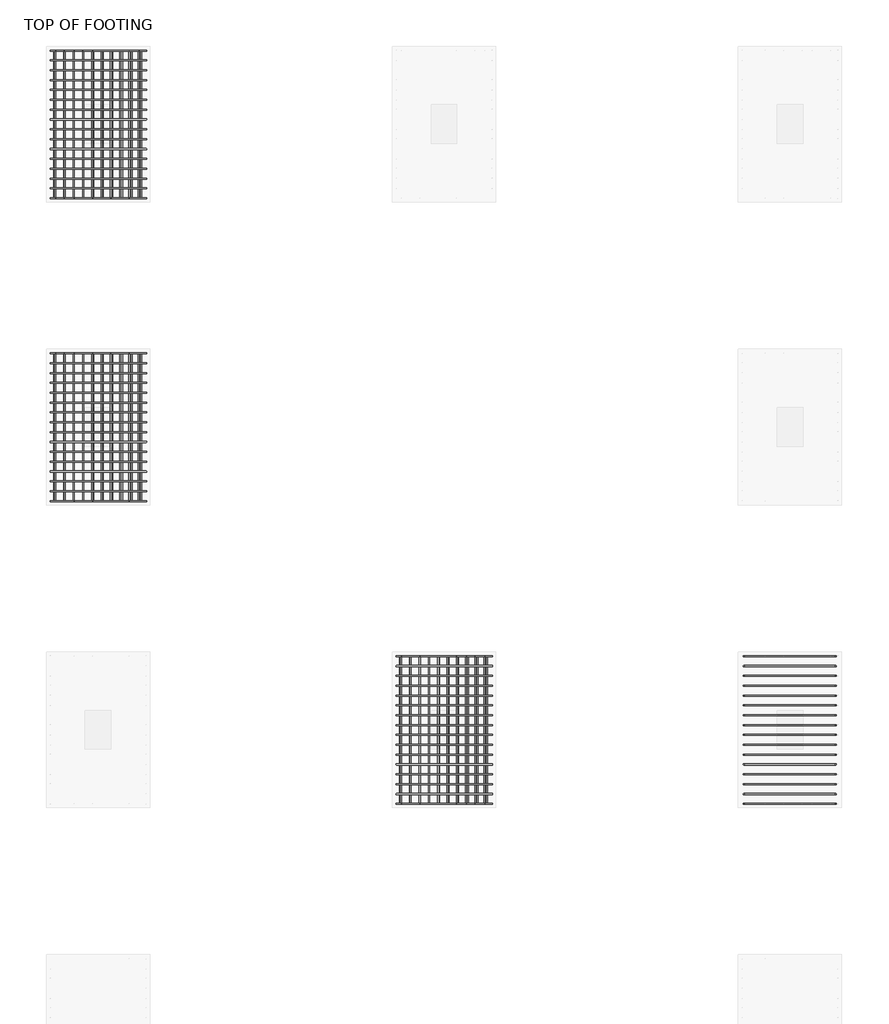
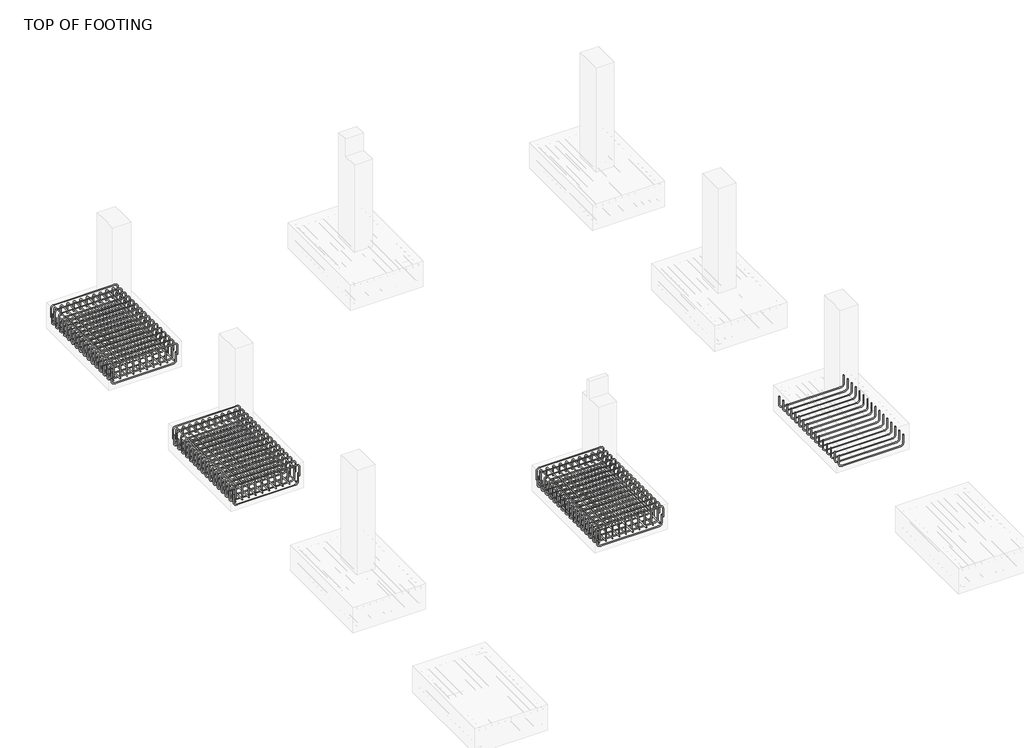
# One storey, part 7 of 8: 13 reinforcing bars.
"""IFC4 building model written with IfcOpenShell, lengths in millimetres."""

from ifc_helpers import new_model, si_unit, point, frame, origin, place, context, project, spatial, polyline, circle_curve, trimmed, segment, composite_curve, source, transform, mapped, element, save
from ifc_brep_helpers import swept_disk

model = new_model("IFC4")

# Units and contexts
model_context = context("Model", 3, world=origin())
ifc_project = project(units=[si_unit("LENGTHUNIT", "METRE", prefix="MILLI")], contexts=[model_context])

# Site, building, storey
site = spatial("IfcSite", under=ifc_project)
building = spatial("IfcBuilding", under=site)
storey = spatial("IfcBuildingStorey", under=building, Name="TOP OF FOOTING", Elevation=-1828.8)

# Reinforcing bars
placement = place(None, origin())
reinforcing_bar_shape = source(origin(), model_context, "Body", "SolidModel", [
    swept_disk(composite_curve([segment(polyline([(4698.4779803, 13126.3508557, -2021.4413313), (4698.4779803, 13126.3508557, -2168.7413313)]), True, "CONTINUOUS"), segment(trimmed(circle_curve(frame((4652.1279803, 13126.3508557, -2168.7413313), z_axis=(0.0, 1.0, 0.0), x_axis=(46.350000000000364, 0.0, 0.0)), 46.35), [point((4698.4779803, 13126.3508557, -2168.7413313))], [point((4652.1279803, 13126.3508557, -2215.0913313))], True, "CARTESIAN"), True, "CONTINUOUS"), segment(polyline([(4652.1279803, 13126.3508557, -2215.0913313), (3679.832969, 13126.3508557, -2215.0913313)]), True, "CONTINUOUS"), segment(trimmed(circle_curve(frame((3679.832969, 13126.3508557, -2168.7413313), z_axis=(0.0, 1.0, 0.0), x_axis=(0.0, 0.0, -46.34999999999991)), 46.35), [point((3679.832969, 13126.3508557, -2215.0913313))], [point((3633.482969, 13126.3508557, -2168.7413313))], True, "CARTESIAN"), True, "CONTINUOUS"), segment(polyline([(3633.482969, 13126.3508557, -2168.7413313), (3633.482969, 13126.3508557, -2021.4413313)]), True, "CONTINUOUS")], self_intersect=False), 6.35),
])
element("IfcReinforcingBar", 1, at=placement, inside=storey, context=model_context, shape_type="MappedRepresentation", body=[
    mapped(reinforcing_bar_shape, transform((0.0, 0.0, 0.0), x_axis=(1.0, 0.0, 0.0), y_axis=(0.0, 1.0, 0.0), z_axis=(0.0, 0.0, 1.0))),
    mapped(reinforcing_bar_shape, transform((0.0, -113.82, 0.0), x_axis=(1.0, 0.0, 0.0), y_axis=(0.0, 1.0, 0.0), z_axis=(0.0, 0.0, 1.0))),
    mapped(reinforcing_bar_shape, transform((0.0, -227.64, 0.0), x_axis=(1.0, 0.0, 0.0), y_axis=(0.0, 1.0, 0.0), z_axis=(0.0, 0.0, 1.0))),
    mapped(reinforcing_bar_shape, transform((0.0, -341.46, 0.0), x_axis=(1.0, 0.0, 0.0), y_axis=(0.0, 1.0, 0.0), z_axis=(0.0, 0.0, 1.0))),
    mapped(reinforcing_bar_shape, transform((0.0, -455.28, 0.0), x_axis=(1.0, 0.0, 0.0), y_axis=(0.0, 1.0, 0.0), z_axis=(0.0, 0.0, 1.0))),
    mapped(reinforcing_bar_shape, transform((0.0, -569.1, 0.0), x_axis=(1.0, 0.0, 0.0), y_axis=(0.0, 1.0, 0.0), z_axis=(0.0, 0.0, 1.0))),
    mapped(reinforcing_bar_shape, transform((0.0, -682.92, 0.0), x_axis=(1.0, 0.0, 0.0), y_axis=(0.0, 1.0, 0.0), z_axis=(0.0, 0.0, 1.0))),
    mapped(reinforcing_bar_shape, transform((0.0, -796.74, 0.0), x_axis=(1.0, 0.0, 0.0), y_axis=(0.0, 1.0, 0.0), z_axis=(0.0, 0.0, 1.0))),
    mapped(reinforcing_bar_shape, transform((0.0, -910.56, 0.0), x_axis=(1.0, 0.0, 0.0), y_axis=(0.0, 1.0, 0.0), z_axis=(0.0, 0.0, 1.0))),
    mapped(reinforcing_bar_shape, transform((0.0, -1024.38, 0.0), x_axis=(1.0, 0.0, 0.0), y_axis=(0.0, 1.0, 0.0), z_axis=(0.0, 0.0, 1.0))),
    mapped(reinforcing_bar_shape, transform((0.0, -1138.2, 0.0), x_axis=(1.0, 0.0, 0.0), y_axis=(0.0, 1.0, 0.0), z_axis=(0.0, 0.0, 1.0))),
    mapped(reinforcing_bar_shape, transform((0.0, -1252.02, 0.0), x_axis=(1.0, 0.0, 0.0), y_axis=(0.0, 1.0, 0.0), z_axis=(0.0, 0.0, 1.0))),
    mapped(reinforcing_bar_shape, transform((0.0, -1365.84, 0.0), x_axis=(1.0, 0.0, 0.0), y_axis=(0.0, 1.0, 0.0), z_axis=(0.0, 0.0, 1.0))),
    mapped(reinforcing_bar_shape, transform((0.0, -1479.66, 0.0), x_axis=(1.0, 0.0, 0.0), y_axis=(0.0, 1.0, 0.0), z_axis=(0.0, 0.0, 1.0))),
    mapped(reinforcing_bar_shape, transform((0.0, -1593.48, 0.0), x_axis=(1.0, 0.0, 0.0), y_axis=(0.0, 1.0, 0.0), z_axis=(0.0, 0.0, 1.0))),
    mapped(reinforcing_bar_shape, transform((0.0, -1707.3, 0.0), x_axis=(1.0, 0.0, 0.0), y_axis=(0.0, 1.0, 0.0), z_axis=(0.0, 0.0, 1.0))),
])
reinforcing_bar_2_shape = source(origin(), model_context, "Body", "SolidModel", [
    swept_disk(composite_curve([segment(polyline([(3615.6625983, 13126.3508557, -2068.8), (3615.6625983, 13126.3508557, -1921.5)]), True, "CONTINUOUS"), segment(trimmed(circle_curve(frame((3662.0125983, 13126.3508557, -1921.5), z_axis=(0.0, 1.0, 0.0), x_axis=(-46.34999999999991, 0.0, 0.0)), 46.35), [point((3615.6625983, 13126.3508557, -1921.5))], [point((3662.0125983, 13126.3508557, -1875.15))], True, "CARTESIAN"), True, "CONTINUOUS"), segment(polyline([(3662.0125983, 13126.3508557, -1875.15), (4676.6125983, 13126.3508557, -1875.15)]), True, "CONTINUOUS"), segment(trimmed(circle_curve(frame((4676.6125983, 13126.3508557, -1921.5), z_axis=(0.0, 1.0, 0.0), x_axis=(0.0, 0.0, 46.34999999999991)), 46.35), [point((4676.6125983, 13126.3508557, -1875.15))], [point((4722.9625983, 13126.3508557, -1921.5))], True, "CARTESIAN"), True, "CONTINUOUS"), segment(polyline([(4722.9625983, 13126.3508557, -1921.5), (4722.9625983, 13126.3508557, -2068.8)]), True, "CONTINUOUS")], self_intersect=False), 6.35),
])
element("IfcReinforcingBar", 2, at=placement, inside=storey, context=model_context, shape_type="MappedRepresentation", body=[
    mapped(reinforcing_bar_2_shape, transform((0.0, 0.0, 0.0), x_axis=(1.0, 0.0, 0.0), y_axis=(0.0, 1.0, 0.0), z_axis=(0.0, 0.0, 1.0))),
    mapped(reinforcing_bar_2_shape, transform((0.0, -113.82, 0.0), x_axis=(1.0, 0.0, 0.0), y_axis=(0.0, 1.0, 0.0), z_axis=(0.0, 0.0, 1.0))),
    mapped(reinforcing_bar_2_shape, transform((0.0, -227.64, 0.0), x_axis=(1.0, 0.0, 0.0), y_axis=(0.0, 1.0, 0.0), z_axis=(0.0, 0.0, 1.0))),
    mapped(reinforcing_bar_2_shape, transform((0.0, -341.46, 0.0), x_axis=(1.0, 0.0, 0.0), y_axis=(0.0, 1.0, 0.0), z_axis=(0.0, 0.0, 1.0))),
    mapped(reinforcing_bar_2_shape, transform((0.0, -455.28, 0.0), x_axis=(1.0, 0.0, 0.0), y_axis=(0.0, 1.0, 0.0), z_axis=(0.0, 0.0, 1.0))),
    mapped(reinforcing_bar_2_shape, transform((0.0, -569.1, 0.0), x_axis=(1.0, 0.0, 0.0), y_axis=(0.0, 1.0, 0.0), z_axis=(0.0, 0.0, 1.0))),
    mapped(reinforcing_bar_2_shape, transform((0.0, -682.92, 0.0), x_axis=(1.0, 0.0, 0.0), y_axis=(0.0, 1.0, 0.0), z_axis=(0.0, 0.0, 1.0))),
    mapped(reinforcing_bar_2_shape, transform((0.0, -796.74, 0.0), x_axis=(1.0, 0.0, 0.0), y_axis=(0.0, 1.0, 0.0), z_axis=(0.0, 0.0, 1.0))),
    mapped(reinforcing_bar_2_shape, transform((0.0, -910.56, 0.0), x_axis=(1.0, 0.0, 0.0), y_axis=(0.0, 1.0, 0.0), z_axis=(0.0, 0.0, 1.0))),
    mapped(reinforcing_bar_2_shape, transform((0.0, -1024.38, 0.0), x_axis=(1.0, 0.0, 0.0), y_axis=(0.0, 1.0, 0.0), z_axis=(0.0, 0.0, 1.0))),
    mapped(reinforcing_bar_2_shape, transform((0.0, -1138.2, 0.0), x_axis=(1.0, 0.0, 0.0), y_axis=(0.0, 1.0, 0.0), z_axis=(0.0, 0.0, 1.0))),
    mapped(reinforcing_bar_2_shape, transform((0.0, -1252.02, 0.0), x_axis=(1.0, 0.0, 0.0), y_axis=(0.0, 1.0, 0.0), z_axis=(0.0, 0.0, 1.0))),
    mapped(reinforcing_bar_2_shape, transform((0.0, -1365.84, 0.0), x_axis=(1.0, 0.0, 0.0), y_axis=(0.0, 1.0, 0.0), z_axis=(0.0, 0.0, 1.0))),
    mapped(reinforcing_bar_2_shape, transform((0.0, -1479.66, 0.0), x_axis=(1.0, 0.0, 0.0), y_axis=(0.0, 1.0, 0.0), z_axis=(0.0, 0.0, 1.0))),
    mapped(reinforcing_bar_2_shape, transform((0.0, -1593.48, 0.0), x_axis=(1.0, 0.0, 0.0), y_axis=(0.0, 1.0, 0.0), z_axis=(0.0, 0.0, 1.0))),
    mapped(reinforcing_bar_2_shape, transform((0.0, -1707.3, 0.0), x_axis=(1.0, 0.0, 0.0), y_axis=(0.0, 1.0, 0.0), z_axis=(0.0, 0.0, 1.0))),
])
reinforcing_bar_3_shape = source(origin(), model_context, "Body", "SolidModel", [
    swept_disk(composite_curve([segment(polyline([(3660.407291, 13132.7008557, -2155.1176129), (3660.407291, 11412.7008557, -2155.1176129)]), True, "CONTINUOUS")], self_intersect=False), 6.35),
])
element("IfcReinforcingBar", 3, at=placement, inside=storey, context=model_context, shape_type="MappedRepresentation", body=[
    mapped(reinforcing_bar_3_shape, transform((0.0, 0.0, 0.0), x_axis=(1.0, 0.0, 0.0), y_axis=(0.0, 1.0, 0.0), z_axis=(0.0, 0.0, 1.0))),
    mapped(reinforcing_bar_3_shape, transform((111.602188, 0.0, 0.0), x_axis=(1.0, 0.0, 0.0), y_axis=(0.0, 1.0, 0.0), z_axis=(0.0, 0.0, 1.0))),
    mapped(reinforcing_bar_3_shape, transform((223.2043759, 0.0, 0.0), x_axis=(1.0, 0.0, 0.0), y_axis=(0.0, 1.0, 0.0), z_axis=(0.0, 0.0, 1.0))),
    mapped(reinforcing_bar_3_shape, transform((334.8065639, 0.0, 0.0), x_axis=(1.0, 0.0, 0.0), y_axis=(0.0, 1.0, 0.0), z_axis=(0.0, 0.0, 1.0))),
    mapped(reinforcing_bar_3_shape, transform((446.4087519, 0.0, 0.0), x_axis=(1.0, 0.0, 0.0), y_axis=(0.0, 1.0, 0.0), z_axis=(0.0, 0.0, 1.0))),
    mapped(reinforcing_bar_3_shape, transform((558.0109398, 0.0, 0.0), x_axis=(1.0, 0.0, 0.0), y_axis=(0.0, 1.0, 0.0), z_axis=(0.0, 0.0, 1.0))),
    mapped(reinforcing_bar_3_shape, transform((669.6131278, 0.0, 0.0), x_axis=(1.0, 0.0, 0.0), y_axis=(0.0, 1.0, 0.0), z_axis=(0.0, 0.0, 1.0))),
    mapped(reinforcing_bar_3_shape, transform((781.2153158, 0.0, 0.0), x_axis=(1.0, 0.0, 0.0), y_axis=(0.0, 1.0, 0.0), z_axis=(0.0, 0.0, 1.0))),
    mapped(reinforcing_bar_3_shape, transform((892.8175037, 0.0, 0.0), x_axis=(1.0, 0.0, 0.0), y_axis=(0.0, 1.0, 0.0), z_axis=(0.0, 0.0, 1.0))),
    mapped(reinforcing_bar_3_shape, transform((1004.4196917, 0.0, 0.0), x_axis=(1.0, 0.0, 0.0), y_axis=(0.0, 1.0, 0.0), z_axis=(0.0, 0.0, 1.0))),
])
reinforcing_bar_4_shape = source(origin(), model_context, "Body", "SolidModel", [
    swept_disk(composite_curve([segment(polyline([(4635.7348019, 13126.3508557, -2094.6521303), (4635.7348019, 13126.3508557, -1947.3521303)]), True, "CONTINUOUS"), segment(trimmed(circle_curve(frame((4635.7348019, 13080.0008557, -1947.3521303), z_axis=(1.0, 0.0, 0.0), x_axis=(0.0, 46.350000000000364, 0.0)), 46.35), [point((4635.7348019, 13126.3508557, -1947.3521303))], [point((4635.7348019, 13080.0008557, -1901.0021303))], True, "CARTESIAN"), True, "CONTINUOUS"), segment(polyline([(4635.7348019, 13080.0008557, -1901.0021303), (4635.7348019, 11465.4008557, -1901.0021303)]), True, "CONTINUOUS"), segment(trimmed(circle_curve(frame((4635.7348019, 11465.4008557, -1947.3521303), z_axis=(1.0, 0.0, 0.0), x_axis=(0.0, 0.0, 46.34999999999991)), 46.35), [point((4635.7348019, 11465.4008557, -1901.0021303))], [point((4635.7348019, 11419.0508557, -1947.3521303))], True, "CARTESIAN"), True, "CONTINUOUS"), segment(polyline([(4635.7348019, 11419.0508557, -1947.3521303), (4635.7348019, 11419.0508557, -2094.6521303)]), True, "CONTINUOUS")], self_intersect=False), 6.35),
])
element("IfcReinforcingBar", 4, at=placement, inside=storey, context=model_context, shape_type="MappedRepresentation", body=[
    mapped(reinforcing_bar_4_shape, transform((0.0, 0.0, 0.0), x_axis=(1.0, 0.0, 0.0), y_axis=(0.0, 1.0, 0.0), z_axis=(0.0, 0.0, 1.0))),
    mapped(reinforcing_bar_4_shape, transform((-107.1680233, 0.0, 0.0), x_axis=(1.0, 0.0, 0.0), y_axis=(0.0, 1.0, 0.0), z_axis=(0.0, 0.0, 1.0))),
    mapped(reinforcing_bar_4_shape, transform((-214.3360466, 0.0, 0.0), x_axis=(1.0, 0.0, 0.0), y_axis=(0.0, 1.0, 0.0), z_axis=(0.0, 0.0, 1.0))),
    mapped(reinforcing_bar_4_shape, transform((-321.5040699, 0.0, 0.0), x_axis=(1.0, 0.0, 0.0), y_axis=(0.0, 1.0, 0.0), z_axis=(0.0, 0.0, 1.0))),
    mapped(reinforcing_bar_4_shape, transform((-428.6720932, 0.0, 0.0), x_axis=(1.0, 0.0, 0.0), y_axis=(0.0, 1.0, 0.0), z_axis=(0.0, 0.0, 1.0))),
    mapped(reinforcing_bar_4_shape, transform((-535.8401165, 0.0, 0.0), x_axis=(1.0, 0.0, 0.0), y_axis=(0.0, 1.0, 0.0), z_axis=(0.0, 0.0, 1.0))),
    mapped(reinforcing_bar_4_shape, transform((-643.0081398, 0.0, 0.0), x_axis=(1.0, 0.0, 0.0), y_axis=(0.0, 1.0, 0.0), z_axis=(0.0, 0.0, 1.0))),
    mapped(reinforcing_bar_4_shape, transform((-750.176163, 0.0, 0.0), x_axis=(1.0, 0.0, 0.0), y_axis=(0.0, 1.0, 0.0), z_axis=(0.0, 0.0, 1.0))),
    mapped(reinforcing_bar_4_shape, transform((-857.3441863, 0.0, 0.0), x_axis=(1.0, 0.0, 0.0), y_axis=(0.0, 1.0, 0.0), z_axis=(0.0, 0.0, 1.0))),
    mapped(reinforcing_bar_4_shape, transform((-964.5122096, 0.0, 0.0), x_axis=(1.0, 0.0, 0.0), y_axis=(0.0, 1.0, 0.0), z_axis=(0.0, 0.0, 1.0))),
])
reinforcing_bar_5_shape = source(origin(), model_context, "Body", "SolidModel", [
    swept_disk(composite_curve([segment(polyline([(4698.4779803, 16626.3508557, -2021.4413313), (4698.4779803, 16626.3508557, -2168.7413313)]), True, "CONTINUOUS"), segment(trimmed(circle_curve(frame((4652.1279803, 16626.3508557, -2168.7413313), z_axis=(0.0, 1.0, 0.0), x_axis=(46.350000000000364, 0.0, 0.0)), 46.35), [point((4698.4779803, 16626.3508557, -2168.7413313))], [point((4652.1279803, 16626.3508557, -2215.0913313))], True, "CARTESIAN"), True, "CONTINUOUS"), segment(polyline([(4652.1279803, 16626.3508557, -2215.0913313), (3679.832969, 16626.3508557, -2215.0913313)]), True, "CONTINUOUS"), segment(trimmed(circle_curve(frame((3679.832969, 16626.3508557, -2168.7413313), z_axis=(0.0, 1.0, 0.0), x_axis=(0.0, 0.0, -46.34999999999991)), 46.35), [point((3679.832969, 16626.3508557, -2215.0913313))], [point((3633.482969, 16626.3508557, -2168.7413313))], True, "CARTESIAN"), True, "CONTINUOUS"), segment(polyline([(3633.482969, 16626.3508557, -2168.7413313), (3633.482969, 16626.3508557, -2021.4413313)]), True, "CONTINUOUS")], self_intersect=False), 6.35),
])
element("IfcReinforcingBar", 5, at=placement, inside=storey, context=model_context, shape_type="MappedRepresentation", body=[
    mapped(reinforcing_bar_5_shape, transform((0.0, 0.0, 0.0), x_axis=(1.0, 0.0, 0.0), y_axis=(0.0, 1.0, 0.0), z_axis=(0.0, 0.0, 1.0))),
    mapped(reinforcing_bar_5_shape, transform((0.0, -113.82, 0.0), x_axis=(1.0, 0.0, 0.0), y_axis=(0.0, 1.0, 0.0), z_axis=(0.0, 0.0, 1.0))),
    mapped(reinforcing_bar_5_shape, transform((0.0, -227.64, 0.0), x_axis=(1.0, 0.0, 0.0), y_axis=(0.0, 1.0, 0.0), z_axis=(0.0, 0.0, 1.0))),
    mapped(reinforcing_bar_5_shape, transform((0.0, -341.46, 0.0), x_axis=(1.0, 0.0, 0.0), y_axis=(0.0, 1.0, 0.0), z_axis=(0.0, 0.0, 1.0))),
    mapped(reinforcing_bar_5_shape, transform((0.0, -455.28, 0.0), x_axis=(1.0, 0.0, 0.0), y_axis=(0.0, 1.0, 0.0), z_axis=(0.0, 0.0, 1.0))),
    mapped(reinforcing_bar_5_shape, transform((0.0, -569.1, 0.0), x_axis=(1.0, 0.0, 0.0), y_axis=(0.0, 1.0, 0.0), z_axis=(0.0, 0.0, 1.0))),
    mapped(reinforcing_bar_5_shape, transform((0.0, -682.92, 0.0), x_axis=(1.0, 0.0, 0.0), y_axis=(0.0, 1.0, 0.0), z_axis=(0.0, 0.0, 1.0))),
    mapped(reinforcing_bar_5_shape, transform((0.0, -796.74, 0.0), x_axis=(1.0, 0.0, 0.0), y_axis=(0.0, 1.0, 0.0), z_axis=(0.0, 0.0, 1.0))),
    mapped(reinforcing_bar_5_shape, transform((0.0, -910.56, 0.0), x_axis=(1.0, 0.0, 0.0), y_axis=(0.0, 1.0, 0.0), z_axis=(0.0, 0.0, 1.0))),
    mapped(reinforcing_bar_5_shape, transform((0.0, -1024.38, 0.0), x_axis=(1.0, 0.0, 0.0), y_axis=(0.0, 1.0, 0.0), z_axis=(0.0, 0.0, 1.0))),
    mapped(reinforcing_bar_5_shape, transform((0.0, -1138.2, 0.0), x_axis=(1.0, 0.0, 0.0), y_axis=(0.0, 1.0, 0.0), z_axis=(0.0, 0.0, 1.0))),
    mapped(reinforcing_bar_5_shape, transform((0.0, -1252.02, 0.0), x_axis=(1.0, 0.0, 0.0), y_axis=(0.0, 1.0, 0.0), z_axis=(0.0, 0.0, 1.0))),
    mapped(reinforcing_bar_5_shape, transform((0.0, -1365.84, 0.0), x_axis=(1.0, 0.0, 0.0), y_axis=(0.0, 1.0, 0.0), z_axis=(0.0, 0.0, 1.0))),
    mapped(reinforcing_bar_5_shape, transform((0.0, -1479.66, 0.0), x_axis=(1.0, 0.0, 0.0), y_axis=(0.0, 1.0, 0.0), z_axis=(0.0, 0.0, 1.0))),
    mapped(reinforcing_bar_5_shape, transform((0.0, -1593.48, 0.0), x_axis=(1.0, 0.0, 0.0), y_axis=(0.0, 1.0, 0.0), z_axis=(0.0, 0.0, 1.0))),
    mapped(reinforcing_bar_5_shape, transform((0.0, -1707.3, 0.0), x_axis=(1.0, 0.0, 0.0), y_axis=(0.0, 1.0, 0.0), z_axis=(0.0, 0.0, 1.0))),
])
reinforcing_bar_6_shape = source(origin(), model_context, "Body", "SolidModel", [
    swept_disk(composite_curve([segment(polyline([(3615.6625983, 16626.3508557, -2068.8), (3615.6625983, 16626.3508557, -1921.5)]), True, "CONTINUOUS"), segment(trimmed(circle_curve(frame((3662.0125983, 16626.3508557, -1921.5), z_axis=(0.0, 1.0, 0.0), x_axis=(-46.34999999999991, 0.0, 0.0)), 46.35), [point((3615.6625983, 16626.3508557, -1921.5))], [point((3662.0125983, 16626.3508557, -1875.15))], True, "CARTESIAN"), True, "CONTINUOUS"), segment(polyline([(3662.0125983, 16626.3508557, -1875.15), (4676.6125983, 16626.3508557, -1875.15)]), True, "CONTINUOUS"), segment(trimmed(circle_curve(frame((4676.6125983, 16626.3508557, -1921.5), z_axis=(0.0, 1.0, 0.0), x_axis=(0.0, 0.0, 46.34999999999991)), 46.35), [point((4676.6125983, 16626.3508557, -1875.15))], [point((4722.9625983, 16626.3508557, -1921.5))], True, "CARTESIAN"), True, "CONTINUOUS"), segment(polyline([(4722.9625983, 16626.3508557, -1921.5), (4722.9625983, 16626.3508557, -2068.8)]), True, "CONTINUOUS")], self_intersect=False), 6.35),
])
element("IfcReinforcingBar", 6, at=placement, inside=storey, context=model_context, shape_type="MappedRepresentation", body=[
    mapped(reinforcing_bar_6_shape, transform((0.0, 0.0, 0.0), x_axis=(1.0, 0.0, 0.0), y_axis=(0.0, 1.0, 0.0), z_axis=(0.0, 0.0, 1.0))),
    mapped(reinforcing_bar_6_shape, transform((0.0, -113.82, 0.0), x_axis=(1.0, 0.0, 0.0), y_axis=(0.0, 1.0, 0.0), z_axis=(0.0, 0.0, 1.0))),
    mapped(reinforcing_bar_6_shape, transform((0.0, -227.64, 0.0), x_axis=(1.0, 0.0, 0.0), y_axis=(0.0, 1.0, 0.0), z_axis=(0.0, 0.0, 1.0))),
    mapped(reinforcing_bar_6_shape, transform((0.0, -341.46, 0.0), x_axis=(1.0, 0.0, 0.0), y_axis=(0.0, 1.0, 0.0), z_axis=(0.0, 0.0, 1.0))),
    mapped(reinforcing_bar_6_shape, transform((0.0, -455.28, 0.0), x_axis=(1.0, 0.0, 0.0), y_axis=(0.0, 1.0, 0.0), z_axis=(0.0, 0.0, 1.0))),
    mapped(reinforcing_bar_6_shape, transform((0.0, -569.1, 0.0), x_axis=(1.0, 0.0, 0.0), y_axis=(0.0, 1.0, 0.0), z_axis=(0.0, 0.0, 1.0))),
    mapped(reinforcing_bar_6_shape, transform((0.0, -682.92, 0.0), x_axis=(1.0, 0.0, 0.0), y_axis=(0.0, 1.0, 0.0), z_axis=(0.0, 0.0, 1.0))),
    mapped(reinforcing_bar_6_shape, transform((0.0, -796.74, 0.0), x_axis=(1.0, 0.0, 0.0), y_axis=(0.0, 1.0, 0.0), z_axis=(0.0, 0.0, 1.0))),
    mapped(reinforcing_bar_6_shape, transform((0.0, -910.56, 0.0), x_axis=(1.0, 0.0, 0.0), y_axis=(0.0, 1.0, 0.0), z_axis=(0.0, 0.0, 1.0))),
    mapped(reinforcing_bar_6_shape, transform((0.0, -1024.38, 0.0), x_axis=(1.0, 0.0, 0.0), y_axis=(0.0, 1.0, 0.0), z_axis=(0.0, 0.0, 1.0))),
    mapped(reinforcing_bar_6_shape, transform((0.0, -1138.2, 0.0), x_axis=(1.0, 0.0, 0.0), y_axis=(0.0, 1.0, 0.0), z_axis=(0.0, 0.0, 1.0))),
    mapped(reinforcing_bar_6_shape, transform((0.0, -1252.02, 0.0), x_axis=(1.0, 0.0, 0.0), y_axis=(0.0, 1.0, 0.0), z_axis=(0.0, 0.0, 1.0))),
    mapped(reinforcing_bar_6_shape, transform((0.0, -1365.84, 0.0), x_axis=(1.0, 0.0, 0.0), y_axis=(0.0, 1.0, 0.0), z_axis=(0.0, 0.0, 1.0))),
    mapped(reinforcing_bar_6_shape, transform((0.0, -1479.66, 0.0), x_axis=(1.0, 0.0, 0.0), y_axis=(0.0, 1.0, 0.0), z_axis=(0.0, 0.0, 1.0))),
    mapped(reinforcing_bar_6_shape, transform((0.0, -1593.48, 0.0), x_axis=(1.0, 0.0, 0.0), y_axis=(0.0, 1.0, 0.0), z_axis=(0.0, 0.0, 1.0))),
    mapped(reinforcing_bar_6_shape, transform((0.0, -1707.3, 0.0), x_axis=(1.0, 0.0, 0.0), y_axis=(0.0, 1.0, 0.0), z_axis=(0.0, 0.0, 1.0))),
])
reinforcing_bar_7_shape = source(origin(), model_context, "Body", "SolidModel", [
    swept_disk(composite_curve([segment(polyline([(3660.407291, 16632.7008557, -2155.1176129), (3660.407291, 14912.7008557, -2155.1176129)]), True, "CONTINUOUS")], self_intersect=False), 6.35),
])
element("IfcReinforcingBar", 7, at=placement, inside=storey, context=model_context, shape_type="MappedRepresentation", body=[
    mapped(reinforcing_bar_7_shape, transform((0.0, 0.0, 0.0), x_axis=(1.0, 0.0, 0.0), y_axis=(0.0, 1.0, 0.0), z_axis=(0.0, 0.0, 1.0))),
    mapped(reinforcing_bar_7_shape, transform((111.602188, 0.0, 0.0), x_axis=(1.0, 0.0, 0.0), y_axis=(0.0, 1.0, 0.0), z_axis=(0.0, 0.0, 1.0))),
    mapped(reinforcing_bar_7_shape, transform((223.2043759, 0.0, 0.0), x_axis=(1.0, 0.0, 0.0), y_axis=(0.0, 1.0, 0.0), z_axis=(0.0, 0.0, 1.0))),
    mapped(reinforcing_bar_7_shape, transform((334.8065639, 0.0, 0.0), x_axis=(1.0, 0.0, 0.0), y_axis=(0.0, 1.0, 0.0), z_axis=(0.0, 0.0, 1.0))),
    mapped(reinforcing_bar_7_shape, transform((446.4087519, 0.0, 0.0), x_axis=(1.0, 0.0, 0.0), y_axis=(0.0, 1.0, 0.0), z_axis=(0.0, 0.0, 1.0))),
    mapped(reinforcing_bar_7_shape, transform((558.0109398, 0.0, 0.0), x_axis=(1.0, 0.0, 0.0), y_axis=(0.0, 1.0, 0.0), z_axis=(0.0, 0.0, 1.0))),
    mapped(reinforcing_bar_7_shape, transform((669.6131278, 0.0, 0.0), x_axis=(1.0, 0.0, 0.0), y_axis=(0.0, 1.0, 0.0), z_axis=(0.0, 0.0, 1.0))),
    mapped(reinforcing_bar_7_shape, transform((781.2153158, 0.0, 0.0), x_axis=(1.0, 0.0, 0.0), y_axis=(0.0, 1.0, 0.0), z_axis=(0.0, 0.0, 1.0))),
    mapped(reinforcing_bar_7_shape, transform((892.8175037, 0.0, 0.0), x_axis=(1.0, 0.0, 0.0), y_axis=(0.0, 1.0, 0.0), z_axis=(0.0, 0.0, 1.0))),
    mapped(reinforcing_bar_7_shape, transform((1004.4196917, 0.0, 0.0), x_axis=(1.0, 0.0, 0.0), y_axis=(0.0, 1.0, 0.0), z_axis=(0.0, 0.0, 1.0))),
])
reinforcing_bar_8_shape = source(origin(), model_context, "Body", "SolidModel", [
    swept_disk(composite_curve([segment(polyline([(4635.7348019, 16626.3508557, -2094.6521303), (4635.7348019, 16626.3508557, -1947.3521303)]), True, "CONTINUOUS"), segment(trimmed(circle_curve(frame((4635.7348019, 16580.0008557, -1947.3521303), z_axis=(1.0, 0.0, 0.0), x_axis=(0.0, 46.349999999998545, 0.0)), 46.35), [point((4635.7348019, 16626.3508557, -1947.3521303))], [point((4635.7348019, 16580.0008557, -1901.0021303))], True, "CARTESIAN"), True, "CONTINUOUS"), segment(polyline([(4635.7348019, 16580.0008557, -1901.0021303), (4635.7348019, 14965.4008557, -1901.0021303)]), True, "CONTINUOUS"), segment(trimmed(circle_curve(frame((4635.7348019, 14965.4008557, -1947.3521303), z_axis=(1.0, 0.0, 0.0), x_axis=(0.0, 0.0, 46.34999999999991)), 46.35), [point((4635.7348019, 14965.4008557, -1901.0021303))], [point((4635.7348019, 14919.0508557, -1947.3521303))], True, "CARTESIAN"), True, "CONTINUOUS"), segment(polyline([(4635.7348019, 14919.0508557, -1947.3521303), (4635.7348019, 14919.0508557, -2094.6521303)]), True, "CONTINUOUS")], self_intersect=False), 6.35),
])
element("IfcReinforcingBar", 8, at=placement, inside=storey, context=model_context, shape_type="MappedRepresentation", body=[
    mapped(reinforcing_bar_8_shape, transform((0.0, 0.0, 0.0), x_axis=(1.0, 0.0, 0.0), y_axis=(0.0, 1.0, 0.0), z_axis=(0.0, 0.0, 1.0))),
    mapped(reinforcing_bar_8_shape, transform((-107.1680233, 0.0, 0.0), x_axis=(1.0, 0.0, 0.0), y_axis=(0.0, 1.0, 0.0), z_axis=(0.0, 0.0, 1.0))),
    mapped(reinforcing_bar_8_shape, transform((-214.3360466, 0.0, 0.0), x_axis=(1.0, 0.0, 0.0), y_axis=(0.0, 1.0, 0.0), z_axis=(0.0, 0.0, 1.0))),
    mapped(reinforcing_bar_8_shape, transform((-321.5040699, 0.0, 0.0), x_axis=(1.0, 0.0, 0.0), y_axis=(0.0, 1.0, 0.0), z_axis=(0.0, 0.0, 1.0))),
    mapped(reinforcing_bar_8_shape, transform((-428.6720932, 0.0, 0.0), x_axis=(1.0, 0.0, 0.0), y_axis=(0.0, 1.0, 0.0), z_axis=(0.0, 0.0, 1.0))),
    mapped(reinforcing_bar_8_shape, transform((-535.8401165, 0.0, 0.0), x_axis=(1.0, 0.0, 0.0), y_axis=(0.0, 1.0, 0.0), z_axis=(0.0, 0.0, 1.0))),
    mapped(reinforcing_bar_8_shape, transform((-643.0081398, 0.0, 0.0), x_axis=(1.0, 0.0, 0.0), y_axis=(0.0, 1.0, 0.0), z_axis=(0.0, 0.0, 1.0))),
    mapped(reinforcing_bar_8_shape, transform((-750.176163, 0.0, 0.0), x_axis=(1.0, 0.0, 0.0), y_axis=(0.0, 1.0, 0.0), z_axis=(0.0, 0.0, 1.0))),
    mapped(reinforcing_bar_8_shape, transform((-857.3441863, 0.0, 0.0), x_axis=(1.0, 0.0, 0.0), y_axis=(0.0, 1.0, 0.0), z_axis=(0.0, 0.0, 1.0))),
    mapped(reinforcing_bar_8_shape, transform((-964.5122096, 0.0, 0.0), x_axis=(1.0, 0.0, 0.0), y_axis=(0.0, 1.0, 0.0), z_axis=(0.0, 0.0, 1.0))),
])
reinforcing_bar_9_shape = source(origin(), model_context, "Body", "SolidModel", [
    swept_disk(composite_curve([segment(polyline([(8698.4779803, 9626.3508557, -2021.4413313), (8698.4779803, 9626.3508557, -2168.7413313)]), True, "CONTINUOUS"), segment(trimmed(circle_curve(frame((8652.1279803, 9626.3508557, -2168.7413313), z_axis=(0.0, 1.0, 0.0), x_axis=(46.350000000000364, 0.0, 0.0)), 46.35), [point((8698.4779803, 9626.3508557, -2168.7413313))], [point((8652.1279803, 9626.3508557, -2215.0913313))], True, "CARTESIAN"), True, "CONTINUOUS"), segment(polyline([(8652.1279803, 9626.3508557, -2215.0913313), (7679.832969, 9626.3508557, -2215.0913313)]), True, "CONTINUOUS"), segment(trimmed(circle_curve(frame((7679.832969, 9626.3508557, -2168.7413313), z_axis=(0.0, 1.0, 0.0), x_axis=(0.0, 0.0, -46.34999999999991)), 46.35), [point((7679.832969, 9626.3508557, -2215.0913313))], [point((7633.482969, 9626.3508557, -2168.7413313))], True, "CARTESIAN"), True, "CONTINUOUS"), segment(polyline([(7633.482969, 9626.3508557, -2168.7413313), (7633.482969, 9626.3508557, -2021.4413313)]), True, "CONTINUOUS")], self_intersect=False), 6.35),
])
element("IfcReinforcingBar", 9, at=placement, inside=storey, context=model_context, shape_type="MappedRepresentation", body=[
    mapped(reinforcing_bar_9_shape, transform((0.0, 0.0, 0.0), x_axis=(1.0, 0.0, 0.0), y_axis=(0.0, 1.0, 0.0), z_axis=(0.0, 0.0, 1.0))),
    mapped(reinforcing_bar_9_shape, transform((0.0, -113.82, 0.0), x_axis=(1.0, 0.0, 0.0), y_axis=(0.0, 1.0, 0.0), z_axis=(0.0, 0.0, 1.0))),
    mapped(reinforcing_bar_9_shape, transform((0.0, -227.64, 0.0), x_axis=(1.0, 0.0, 0.0), y_axis=(0.0, 1.0, 0.0), z_axis=(0.0, 0.0, 1.0))),
    mapped(reinforcing_bar_9_shape, transform((0.0, -341.46, 0.0), x_axis=(1.0, 0.0, 0.0), y_axis=(0.0, 1.0, 0.0), z_axis=(0.0, 0.0, 1.0))),
    mapped(reinforcing_bar_9_shape, transform((0.0, -455.28, 0.0), x_axis=(1.0, 0.0, 0.0), y_axis=(0.0, 1.0, 0.0), z_axis=(0.0, 0.0, 1.0))),
    mapped(reinforcing_bar_9_shape, transform((0.0, -569.1, 0.0), x_axis=(1.0, 0.0, 0.0), y_axis=(0.0, 1.0, 0.0), z_axis=(0.0, 0.0, 1.0))),
    mapped(reinforcing_bar_9_shape, transform((0.0, -682.92, 0.0), x_axis=(1.0, 0.0, 0.0), y_axis=(0.0, 1.0, 0.0), z_axis=(0.0, 0.0, 1.0))),
    mapped(reinforcing_bar_9_shape, transform((0.0, -796.74, 0.0), x_axis=(1.0, 0.0, 0.0), y_axis=(0.0, 1.0, 0.0), z_axis=(0.0, 0.0, 1.0))),
    mapped(reinforcing_bar_9_shape, transform((0.0, -910.56, 0.0), x_axis=(1.0, 0.0, 0.0), y_axis=(0.0, 1.0, 0.0), z_axis=(0.0, 0.0, 1.0))),
    mapped(reinforcing_bar_9_shape, transform((0.0, -1024.38, 0.0), x_axis=(1.0, 0.0, 0.0), y_axis=(0.0, 1.0, 0.0), z_axis=(0.0, 0.0, 1.0))),
    mapped(reinforcing_bar_9_shape, transform((0.0, -1138.2, 0.0), x_axis=(1.0, 0.0, 0.0), y_axis=(0.0, 1.0, 0.0), z_axis=(0.0, 0.0, 1.0))),
    mapped(reinforcing_bar_9_shape, transform((0.0, -1252.02, 0.0), x_axis=(1.0, 0.0, 0.0), y_axis=(0.0, 1.0, 0.0), z_axis=(0.0, 0.0, 1.0))),
    mapped(reinforcing_bar_9_shape, transform((0.0, -1365.84, 0.0), x_axis=(1.0, 0.0, 0.0), y_axis=(0.0, 1.0, 0.0), z_axis=(0.0, 0.0, 1.0))),
    mapped(reinforcing_bar_9_shape, transform((0.0, -1479.66, 0.0), x_axis=(1.0, 0.0, 0.0), y_axis=(0.0, 1.0, 0.0), z_axis=(0.0, 0.0, 1.0))),
    mapped(reinforcing_bar_9_shape, transform((0.0, -1593.48, 0.0), x_axis=(1.0, 0.0, 0.0), y_axis=(0.0, 1.0, 0.0), z_axis=(0.0, 0.0, 1.0))),
    mapped(reinforcing_bar_9_shape, transform((0.0, -1707.3, 0.0), x_axis=(1.0, 0.0, 0.0), y_axis=(0.0, 1.0, 0.0), z_axis=(0.0, 0.0, 1.0))),
])
reinforcing_bar_10_shape = source(origin(), model_context, "Body", "SolidModel", [
    swept_disk(composite_curve([segment(polyline([(7615.6625983, 9626.3508557, -2068.8), (7615.6625983, 9626.3508557, -1921.5)]), True, "CONTINUOUS"), segment(trimmed(circle_curve(frame((7662.0125983, 9626.3508557, -1921.5), z_axis=(0.0, 1.0, 0.0), x_axis=(-46.349999999999454, 0.0, 0.0)), 46.35), [point((7615.6625983, 9626.3508557, -1921.5))], [point((7662.0125983, 9626.3508557, -1875.15))], True, "CARTESIAN"), True, "CONTINUOUS"), segment(polyline([(7662.0125983, 9626.3508557, -1875.15), (8676.6125983, 9626.3508557, -1875.15)]), True, "CONTINUOUS"), segment(trimmed(circle_curve(frame((8676.6125983, 9626.3508557, -1921.5), z_axis=(0.0, 1.0, 0.0), x_axis=(0.0, 0.0, 46.34999999999991)), 46.35), [point((8676.6125983, 9626.3508557, -1875.15))], [point((8722.9625983, 9626.3508557, -1921.5))], True, "CARTESIAN"), True, "CONTINUOUS"), segment(polyline([(8722.9625983, 9626.3508557, -1921.5), (8722.9625983, 9626.3508557, -2068.8)]), True, "CONTINUOUS")], self_intersect=False), 6.35),
])
element("IfcReinforcingBar", 10, at=placement, inside=storey, context=model_context, shape_type="MappedRepresentation", body=[
    mapped(reinforcing_bar_10_shape, transform((0.0, 0.0, 0.0), x_axis=(1.0, 0.0, 0.0), y_axis=(0.0, 1.0, 0.0), z_axis=(0.0, 0.0, 1.0))),
    mapped(reinforcing_bar_10_shape, transform((0.0, -113.82, 0.0), x_axis=(1.0, 0.0, 0.0), y_axis=(0.0, 1.0, 0.0), z_axis=(0.0, 0.0, 1.0))),
    mapped(reinforcing_bar_10_shape, transform((0.0, -227.64, 0.0), x_axis=(1.0, 0.0, 0.0), y_axis=(0.0, 1.0, 0.0), z_axis=(0.0, 0.0, 1.0))),
    mapped(reinforcing_bar_10_shape, transform((0.0, -341.46, 0.0), x_axis=(1.0, 0.0, 0.0), y_axis=(0.0, 1.0, 0.0), z_axis=(0.0, 0.0, 1.0))),
    mapped(reinforcing_bar_10_shape, transform((0.0, -455.28, 0.0), x_axis=(1.0, 0.0, 0.0), y_axis=(0.0, 1.0, 0.0), z_axis=(0.0, 0.0, 1.0))),
    mapped(reinforcing_bar_10_shape, transform((0.0, -569.1, 0.0), x_axis=(1.0, 0.0, 0.0), y_axis=(0.0, 1.0, 0.0), z_axis=(0.0, 0.0, 1.0))),
    mapped(reinforcing_bar_10_shape, transform((0.0, -682.92, 0.0), x_axis=(1.0, 0.0, 0.0), y_axis=(0.0, 1.0, 0.0), z_axis=(0.0, 0.0, 1.0))),
    mapped(reinforcing_bar_10_shape, transform((0.0, -796.74, 0.0), x_axis=(1.0, 0.0, 0.0), y_axis=(0.0, 1.0, 0.0), z_axis=(0.0, 0.0, 1.0))),
    mapped(reinforcing_bar_10_shape, transform((0.0, -910.56, 0.0), x_axis=(1.0, 0.0, 0.0), y_axis=(0.0, 1.0, 0.0), z_axis=(0.0, 0.0, 1.0))),
    mapped(reinforcing_bar_10_shape, transform((0.0, -1024.38, 0.0), x_axis=(1.0, 0.0, 0.0), y_axis=(0.0, 1.0, 0.0), z_axis=(0.0, 0.0, 1.0))),
    mapped(reinforcing_bar_10_shape, transform((0.0, -1138.2, 0.0), x_axis=(1.0, 0.0, 0.0), y_axis=(0.0, 1.0, 0.0), z_axis=(0.0, 0.0, 1.0))),
    mapped(reinforcing_bar_10_shape, transform((0.0, -1252.02, 0.0), x_axis=(1.0, 0.0, 0.0), y_axis=(0.0, 1.0, 0.0), z_axis=(0.0, 0.0, 1.0))),
    mapped(reinforcing_bar_10_shape, transform((0.0, -1365.84, 0.0), x_axis=(1.0, 0.0, 0.0), y_axis=(0.0, 1.0, 0.0), z_axis=(0.0, 0.0, 1.0))),
    mapped(reinforcing_bar_10_shape, transform((0.0, -1479.66, 0.0), x_axis=(1.0, 0.0, 0.0), y_axis=(0.0, 1.0, 0.0), z_axis=(0.0, 0.0, 1.0))),
    mapped(reinforcing_bar_10_shape, transform((0.0, -1593.48, 0.0), x_axis=(1.0, 0.0, 0.0), y_axis=(0.0, 1.0, 0.0), z_axis=(0.0, 0.0, 1.0))),
    mapped(reinforcing_bar_10_shape, transform((0.0, -1707.3, 0.0), x_axis=(1.0, 0.0, 0.0), y_axis=(0.0, 1.0, 0.0), z_axis=(0.0, 0.0, 1.0))),
])
reinforcing_bar_11_shape = source(origin(), model_context, "Body", "SolidModel", [
    swept_disk(composite_curve([segment(polyline([(7660.407291, 9632.7008557, -2155.1176129), (7660.407291, 7912.7008557, -2155.1176129)]), True, "CONTINUOUS")], self_intersect=False), 6.35),
])
element("IfcReinforcingBar", 11, at=placement, inside=storey, context=model_context, shape_type="MappedRepresentation", body=[
    mapped(reinforcing_bar_11_shape, transform((0.0, 0.0, 0.0), x_axis=(1.0, 0.0, 0.0), y_axis=(0.0, 1.0, 0.0), z_axis=(0.0, 0.0, 1.0))),
    mapped(reinforcing_bar_11_shape, transform((111.602188, 0.0, 0.0), x_axis=(1.0, 0.0, 0.0), y_axis=(0.0, 1.0, 0.0), z_axis=(0.0, 0.0, 1.0))),
    mapped(reinforcing_bar_11_shape, transform((223.2043759, 0.0, 0.0), x_axis=(1.0, 0.0, 0.0), y_axis=(0.0, 1.0, 0.0), z_axis=(0.0, 0.0, 1.0))),
    mapped(reinforcing_bar_11_shape, transform((334.8065639, 0.0, 0.0), x_axis=(1.0, 0.0, 0.0), y_axis=(0.0, 1.0, 0.0), z_axis=(0.0, 0.0, 1.0))),
    mapped(reinforcing_bar_11_shape, transform((446.4087519, 0.0, 0.0), x_axis=(1.0, 0.0, 0.0), y_axis=(0.0, 1.0, 0.0), z_axis=(0.0, 0.0, 1.0))),
    mapped(reinforcing_bar_11_shape, transform((558.0109398, 0.0, 0.0), x_axis=(1.0, 0.0, 0.0), y_axis=(0.0, 1.0, 0.0), z_axis=(0.0, 0.0, 1.0))),
    mapped(reinforcing_bar_11_shape, transform((669.6131278, 0.0, 0.0), x_axis=(1.0, 0.0, 0.0), y_axis=(0.0, 1.0, 0.0), z_axis=(0.0, 0.0, 1.0))),
    mapped(reinforcing_bar_11_shape, transform((781.2153158, 0.0, 0.0), x_axis=(1.0, 0.0, 0.0), y_axis=(0.0, 1.0, 0.0), z_axis=(0.0, 0.0, 1.0))),
    mapped(reinforcing_bar_11_shape, transform((892.8175037, 0.0, 0.0), x_axis=(1.0, 0.0, 0.0), y_axis=(0.0, 1.0, 0.0), z_axis=(0.0, 0.0, 1.0))),
    mapped(reinforcing_bar_11_shape, transform((1004.4196917, 0.0, 0.0), x_axis=(1.0, 0.0, 0.0), y_axis=(0.0, 1.0, 0.0), z_axis=(0.0, 0.0, 1.0))),
])
reinforcing_bar_12_shape = source(origin(), model_context, "Body", "SolidModel", [
    swept_disk(composite_curve([segment(polyline([(8635.7348019, 9626.3508557, -2094.6521303), (8635.7348019, 9626.3508557, -1947.3521303)]), True, "CONTINUOUS"), segment(trimmed(circle_curve(frame((8635.7348019, 9580.0008557, -1947.3521303), z_axis=(1.0, 0.0, 0.0), x_axis=(0.0, 46.350000000000364, 0.0)), 46.35), [point((8635.7348019, 9626.3508557, -1947.3521303))], [point((8635.7348019, 9580.0008557, -1901.0021303))], True, "CARTESIAN"), True, "CONTINUOUS"), segment(polyline([(8635.7348019, 9580.0008557, -1901.0021303), (8635.7348019, 7965.4008557, -1901.0021303)]), True, "CONTINUOUS"), segment(trimmed(circle_curve(frame((8635.7348019, 7965.4008557, -1947.3521303), z_axis=(1.0, 0.0, 0.0), x_axis=(0.0, 0.0, 46.34999999999991)), 46.35), [point((8635.7348019, 7965.4008557, -1901.0021303))], [point((8635.7348019, 7919.0508557, -1947.3521303))], True, "CARTESIAN"), True, "CONTINUOUS"), segment(polyline([(8635.7348019, 7919.0508557, -1947.3521303), (8635.7348019, 7919.0508557, -2094.6521303)]), True, "CONTINUOUS")], self_intersect=False), 6.35),
])
element("IfcReinforcingBar", 12, at=placement, inside=storey, context=model_context, shape_type="MappedRepresentation", body=[
    mapped(reinforcing_bar_12_shape, transform((0.0, 0.0, 0.0), x_axis=(1.0, 0.0, 0.0), y_axis=(0.0, 1.0, 0.0), z_axis=(0.0, 0.0, 1.0))),
    mapped(reinforcing_bar_12_shape, transform((-107.1680233, 0.0, 0.0), x_axis=(1.0, 0.0, 0.0), y_axis=(0.0, 1.0, 0.0), z_axis=(0.0, 0.0, 1.0))),
    mapped(reinforcing_bar_12_shape, transform((-214.3360466, 0.0, 0.0), x_axis=(1.0, 0.0, 0.0), y_axis=(0.0, 1.0, 0.0), z_axis=(0.0, 0.0, 1.0))),
    mapped(reinforcing_bar_12_shape, transform((-321.5040699, 0.0, 0.0), x_axis=(1.0, 0.0, 0.0), y_axis=(0.0, 1.0, 0.0), z_axis=(0.0, 0.0, 1.0))),
    mapped(reinforcing_bar_12_shape, transform((-428.6720932, 0.0, 0.0), x_axis=(1.0, 0.0, 0.0), y_axis=(0.0, 1.0, 0.0), z_axis=(0.0, 0.0, 1.0))),
    mapped(reinforcing_bar_12_shape, transform((-535.8401165, 0.0, 0.0), x_axis=(1.0, 0.0, 0.0), y_axis=(0.0, 1.0, 0.0), z_axis=(0.0, 0.0, 1.0))),
    mapped(reinforcing_bar_12_shape, transform((-643.0081398, 0.0, 0.0), x_axis=(1.0, 0.0, 0.0), y_axis=(0.0, 1.0, 0.0), z_axis=(0.0, 0.0, 1.0))),
    mapped(reinforcing_bar_12_shape, transform((-750.176163, 0.0, 0.0), x_axis=(1.0, 0.0, 0.0), y_axis=(0.0, 1.0, 0.0), z_axis=(0.0, 0.0, 1.0))),
    mapped(reinforcing_bar_12_shape, transform((-857.3441863, 0.0, 0.0), x_axis=(1.0, 0.0, 0.0), y_axis=(0.0, 1.0, 0.0), z_axis=(0.0, 0.0, 1.0))),
    mapped(reinforcing_bar_12_shape, transform((-964.5122096, 0.0, 0.0), x_axis=(1.0, 0.0, 0.0), y_axis=(0.0, 1.0, 0.0), z_axis=(0.0, 0.0, 1.0))),
])
reinforcing_bar_13_shape = source(origin(), model_context, "Body", "SolidModel", [
    swept_disk(composite_curve([segment(polyline([(12698.4779803, 9626.3508557, -2021.4413313), (12698.4779803, 9626.3508557, -2168.7413313)]), True, "CONTINUOUS"), segment(trimmed(circle_curve(frame((12652.1279803, 9626.3508557, -2168.7413313), z_axis=(0.0, 1.0, 0.0), x_axis=(46.350000000000364, 0.0, 0.0)), 46.35), [point((12698.4779803, 9626.3508557, -2168.7413313))], [point((12652.1279803, 9626.3508557, -2215.0913313))], True, "CARTESIAN"), True, "CONTINUOUS"), segment(polyline([(12652.1279803, 9626.3508557, -2215.0913313), (11679.832969, 9626.3508557, -2215.0913313)]), True, "CONTINUOUS"), segment(trimmed(circle_curve(frame((11679.832969, 9626.3508557, -2168.7413313), z_axis=(0.0, 1.0, 0.0), x_axis=(0.0, 0.0, -46.34999999999991)), 46.35), [point((11679.832969, 9626.3508557, -2215.0913313))], [point((11633.482969, 9626.3508557, -2168.7413313))], True, "CARTESIAN"), True, "CONTINUOUS"), segment(polyline([(11633.482969, 9626.3508557, -2168.7413313), (11633.482969, 9626.3508557, -2021.4413313)]), True, "CONTINUOUS")], self_intersect=False), 6.35),
])
element("IfcReinforcingBar", 13, at=placement, inside=storey, context=model_context, shape_type="MappedRepresentation", body=[
    mapped(reinforcing_bar_13_shape, transform((0.0, 0.0, 0.0), x_axis=(1.0, 0.0, 0.0), y_axis=(0.0, 1.0, 0.0), z_axis=(0.0, 0.0, 1.0))),
    mapped(reinforcing_bar_13_shape, transform((0.0, -113.82, 0.0), x_axis=(1.0, 0.0, 0.0), y_axis=(0.0, 1.0, 0.0), z_axis=(0.0, 0.0, 1.0))),
    mapped(reinforcing_bar_13_shape, transform((0.0, -227.64, 0.0), x_axis=(1.0, 0.0, 0.0), y_axis=(0.0, 1.0, 0.0), z_axis=(0.0, 0.0, 1.0))),
    mapped(reinforcing_bar_13_shape, transform((0.0, -341.46, 0.0), x_axis=(1.0, 0.0, 0.0), y_axis=(0.0, 1.0, 0.0), z_axis=(0.0, 0.0, 1.0))),
    mapped(reinforcing_bar_13_shape, transform((0.0, -455.28, 0.0), x_axis=(1.0, 0.0, 0.0), y_axis=(0.0, 1.0, 0.0), z_axis=(0.0, 0.0, 1.0))),
    mapped(reinforcing_bar_13_shape, transform((0.0, -569.1, 0.0), x_axis=(1.0, 0.0, 0.0), y_axis=(0.0, 1.0, 0.0), z_axis=(0.0, 0.0, 1.0))),
    mapped(reinforcing_bar_13_shape, transform((0.0, -682.92, 0.0), x_axis=(1.0, 0.0, 0.0), y_axis=(0.0, 1.0, 0.0), z_axis=(0.0, 0.0, 1.0))),
    mapped(reinforcing_bar_13_shape, transform((0.0, -796.74, 0.0), x_axis=(1.0, 0.0, 0.0), y_axis=(0.0, 1.0, 0.0), z_axis=(0.0, 0.0, 1.0))),
    mapped(reinforcing_bar_13_shape, transform((0.0, -910.56, 0.0), x_axis=(1.0, 0.0, 0.0), y_axis=(0.0, 1.0, 0.0), z_axis=(0.0, 0.0, 1.0))),
    mapped(reinforcing_bar_13_shape, transform((0.0, -1024.38, 0.0), x_axis=(1.0, 0.0, 0.0), y_axis=(0.0, 1.0, 0.0), z_axis=(0.0, 0.0, 1.0))),
    mapped(reinforcing_bar_13_shape, transform((0.0, -1138.2, 0.0), x_axis=(1.0, 0.0, 0.0), y_axis=(0.0, 1.0, 0.0), z_axis=(0.0, 0.0, 1.0))),
    mapped(reinforcing_bar_13_shape, transform((0.0, -1252.02, 0.0), x_axis=(1.0, 0.0, 0.0), y_axis=(0.0, 1.0, 0.0), z_axis=(0.0, 0.0, 1.0))),
    mapped(reinforcing_bar_13_shape, transform((0.0, -1365.84, 0.0), x_axis=(1.0, 0.0, 0.0), y_axis=(0.0, 1.0, 0.0), z_axis=(0.0, 0.0, 1.0))),
    mapped(reinforcing_bar_13_shape, transform((0.0, -1479.66, 0.0), x_axis=(1.0, 0.0, 0.0), y_axis=(0.0, 1.0, 0.0), z_axis=(0.0, 0.0, 1.0))),
    mapped(reinforcing_bar_13_shape, transform((0.0, -1593.48, 0.0), x_axis=(1.0, 0.0, 0.0), y_axis=(0.0, 1.0, 0.0), z_axis=(0.0, 0.0, 1.0))),
    mapped(reinforcing_bar_13_shape, transform((0.0, -1707.3, 0.0), x_axis=(1.0, 0.0, 0.0), y_axis=(0.0, 1.0, 0.0), z_axis=(0.0, 0.0, 1.0))),
])

save(model, "model.ifc")

# Revit data of these elements
# Elements 1, 2, 3, 4, 5, 6, 7, 8, 9, 10, 11, 12, 13 (IfcReinforcingBar)
#   Phase Created = New Construction
